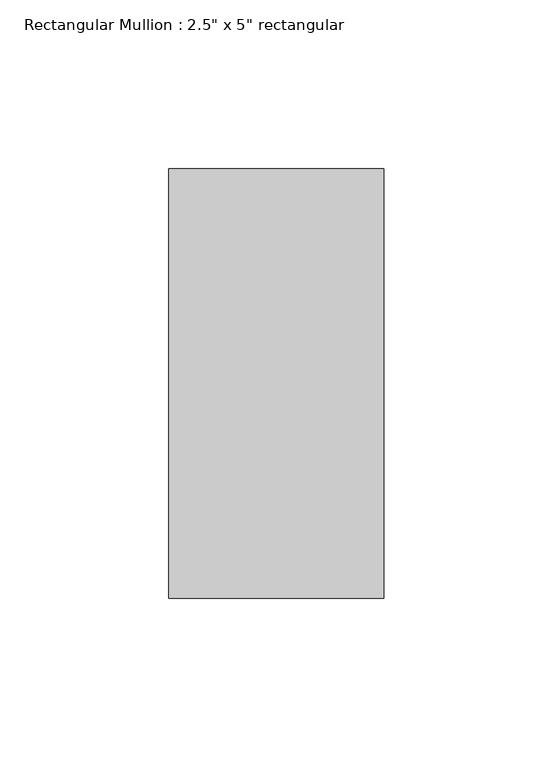
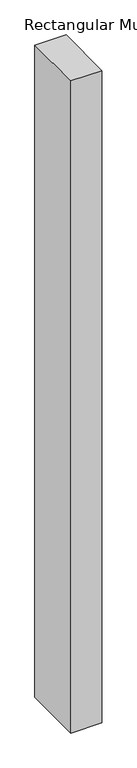
"""IFC4 building model written with IfcOpenShell, lengths in millimetres: member geometry."""

from ifc_helpers import new_model, si_unit, frame, origin, place, context, project, spatial, polyline, outline, extrude, source, transform, mapped, element, save


def member_3bd69304(model_context):
    return source(origin(), model_context, "Body", "SweptSolid", [
        extrude(outline(polyline([(31.75, 63.5), (31.75, -63.5), (-31.75, -63.5), (-31.75, 63.5), (31.75, 63.5)])), frame((0.0, 0.0, -1406.4174829), z_axis=(0.0, 0.0, 1.0), x_axis=(1.0, 0.0, 0.0)), (0.0, 0.0, 1.0), 1406.4174829),
    ])


if __name__ == "__main__":
    model = new_model("IFC4")
    model_context = context("Model", 3, world=origin())
    ifc_project = project(units=[si_unit("LENGTHUNIT", "METRE", prefix="MILLI")], contexts=[model_context])
    site = spatial("IfcSite", under=ifc_project)
    building = spatial("IfcBuilding", under=site)
    placement = place(None, origin())
    member_shape = member_3bd69304(model_context)
    element("IfcMember", 1, ObjectType="Rectangular Mullion : 2.5\" x 5\" rectangular", at=placement, inside=building, context=model_context, shape_type="MappedRepresentation", body=[
        mapped(member_shape, transform((0.0, 0.0, 0.0), x_axis=(1.0, 0.0, 0.0), y_axis=(0.0, 1.0, 0.0), z_axis=(0.0, 0.0, 1.0))),
    ])
    save(model, "model.ifc")

# Revit data of these elements
# Type "Rectangular Mullion : 2.5\" x 5\" rectangular"
#   built-in parameter 1007304 = 0.416667 (stored number, unit not read)
#   built-in parameter 1007301 = 0.104167 (stored number, unit not read)
#   built-in parameter 1007300 = 0.104167 (stored number, unit not read)
# Element 1 (IfcMember, "Rectangular Mullion : 2.5\" x 5\" rectangular")
#   Materials on its faces: "Aluminum"
# Materials
#   "Aluminum": class "Metal", colour RGB 247 247 247, transparency 0, Description = "Aluminum 6061", Cost = 0
